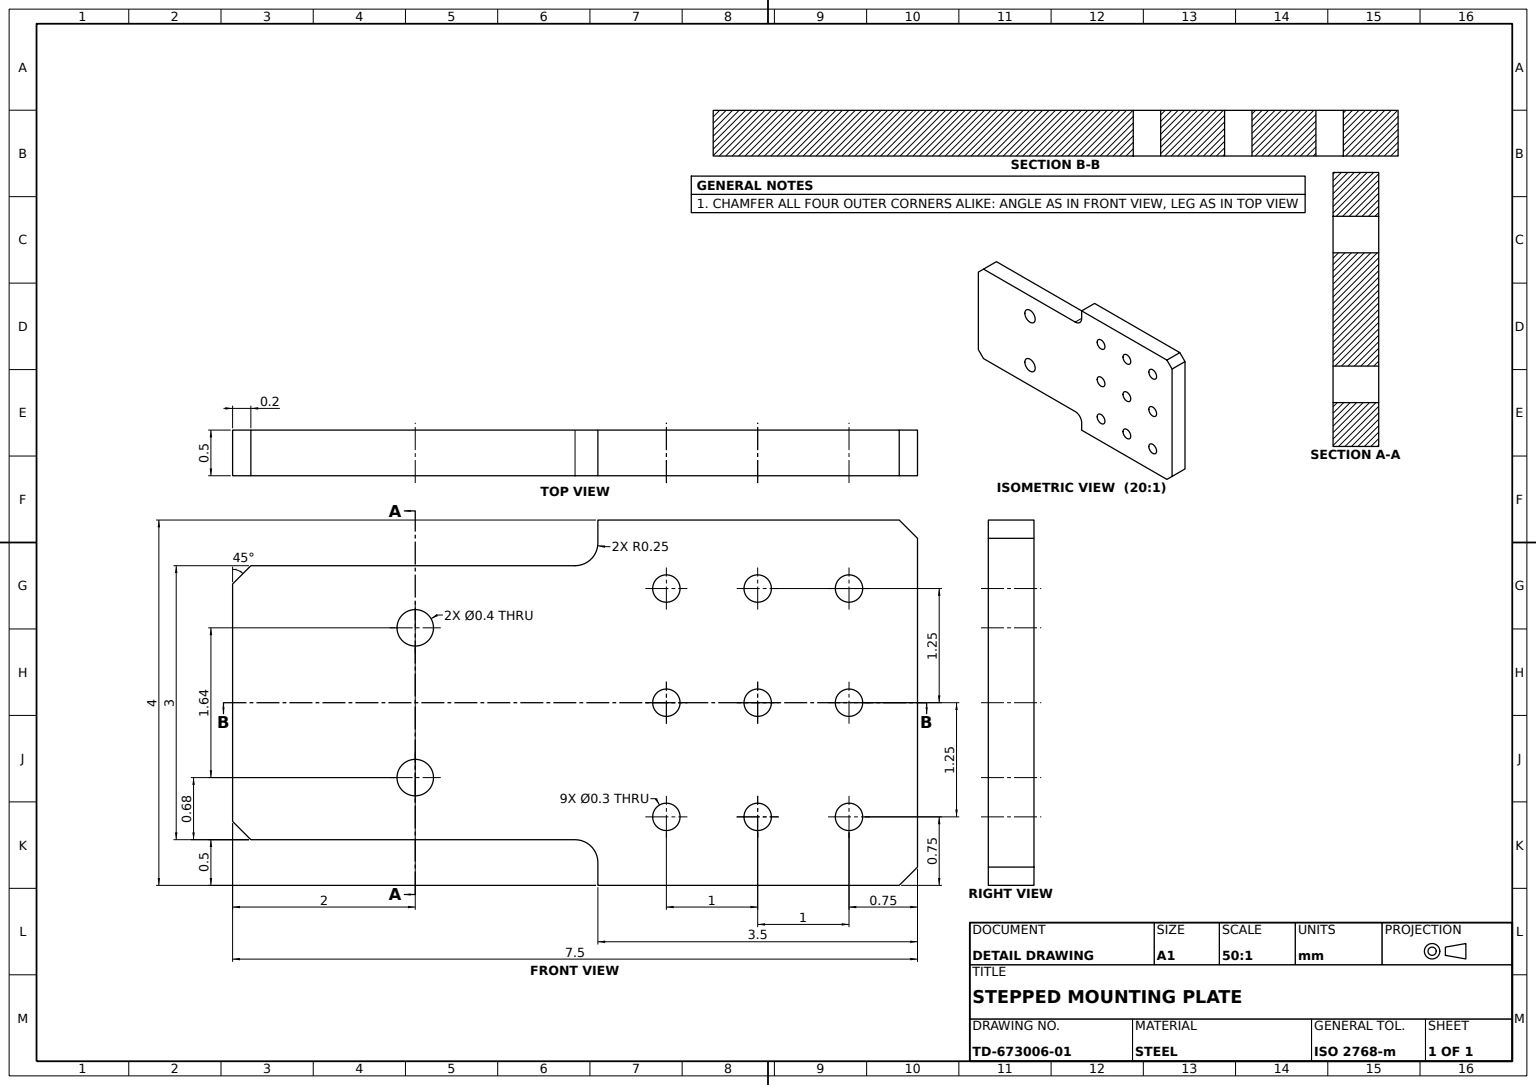
from build123d import *

# Parameters (mm, degrees)
STEPPED_TAB_PLATE_0_5MM_DEPTH = 0.5
CORNER_CHAMFER_0_2X45_A_SIZE  = 0.2
CORNER_CHAMFER_0_2X45_B_SIZE  = 0.2
SCREW_HOLES_SKETCH_R          = 0.2
SCREW_HOLES_2X_DEPTH          = 1
HOLE_GRID_SKETCH_R            = 0.15
HOLE_GRID_3X3_DEPTH           = 1


with BuildPart() as part:
    # Stepped Tab Profile Sketch → Stepped Tab Plate 0.5mm (new body)
    with BuildSketch(Plane.XY):
        with BuildLine():
            ThreePointArc((3.75, 1.5), (3.926776695, 1.573223305), (4, 1.75))
            Line((4, 1.75), (4, 2))
            Line((4, 2), (7.5, 2))
            Line((7.5, 2), (7.5, 0))
            Line((7.5, 0), (0, 0))
            Line((0, 0), (0, 1.5))
            Line((0, 1.5), (3.75, 1.5))
        make_face()
        with BuildLine():
            ThreePointArc((4, -1.75), (3.926776695, -1.573223305), (3.75, -1.5))
            Line((3.75, -1.5), (0, -1.5))
            Line((0, -1.5), (0, 0))
            Line((0, 0), (7.5, 0))
            Line((7.5, 0), (7.5, -2))
            Line((7.5, -2), (4, -2))
            Line((4, -2), (4, -1.75))
        make_face()
    extrude(amount=STEPPED_TAB_PLATE_0_5MM_DEPTH)

    # Corner Chamfer 0.2x45 A
    corner_chamfer_0_2x45_a_edges = [part.edges().sort_by_distance(p)[0] for p in [
        (7.5, 2, 0.25),
        (0, 1.5, 0.25),
    ]]
    chamfer(corner_chamfer_0_2x45_a_edges, length=CORNER_CHAMFER_0_2X45_A_SIZE)

    # Corner Chamfer 0.2x45 B
    corner_chamfer_0_2x45_b_edges = [part.edges().sort_by_distance(p)[0] for p in [
        (7.5, -2, 0.25),
        (0, -1.5, 0.25),
    ]]
    chamfer(corner_chamfer_0_2x45_b_edges, length=CORNER_CHAMFER_0_2X45_B_SIZE)

    # Screw Holes Sketch → Screw Holes 2x (cut)
    with BuildSketch(Plane.XY.offset(0.5)):
        with Locations((2, 0.82)):
            Circle(SCREW_HOLES_SKETCH_R)
        with Locations((2, -0.82)):
            Circle(SCREW_HOLES_SKETCH_R)
    extrude(amount=-SCREW_HOLES_2X_DEPTH, mode=Mode.SUBTRACT)

    # Hole Grid Sketch → Hole Grid 3x3 (cut)
    with BuildSketch(Plane.XY.offset(0.5)):
        with Locations((4.75, 1.25)):
            Circle(HOLE_GRID_SKETCH_R)
        with Locations((5.75, 1.25)):
            Circle(HOLE_GRID_SKETCH_R)
        with Locations((6.75, 1.25)):
            Circle(HOLE_GRID_SKETCH_R)
        with Locations((6.75, 0)):
            Circle(HOLE_GRID_SKETCH_R)
        with Locations((6.75, -1.25)):
            Circle(HOLE_GRID_SKETCH_R)
        with Locations((5.75, -1.25)):
            Circle(HOLE_GRID_SKETCH_R)
        with Locations((4.75, -1.25)):
            Circle(HOLE_GRID_SKETCH_R)
        with Locations((4.75, 0)):
            Circle(HOLE_GRID_SKETCH_R)
        with Locations((5.75, 0)):
            Circle(HOLE_GRID_SKETCH_R)
    extrude(amount=-HOLE_GRID_3X3_DEPTH, mode=Mode.SUBTRACT)


solid = part.part
